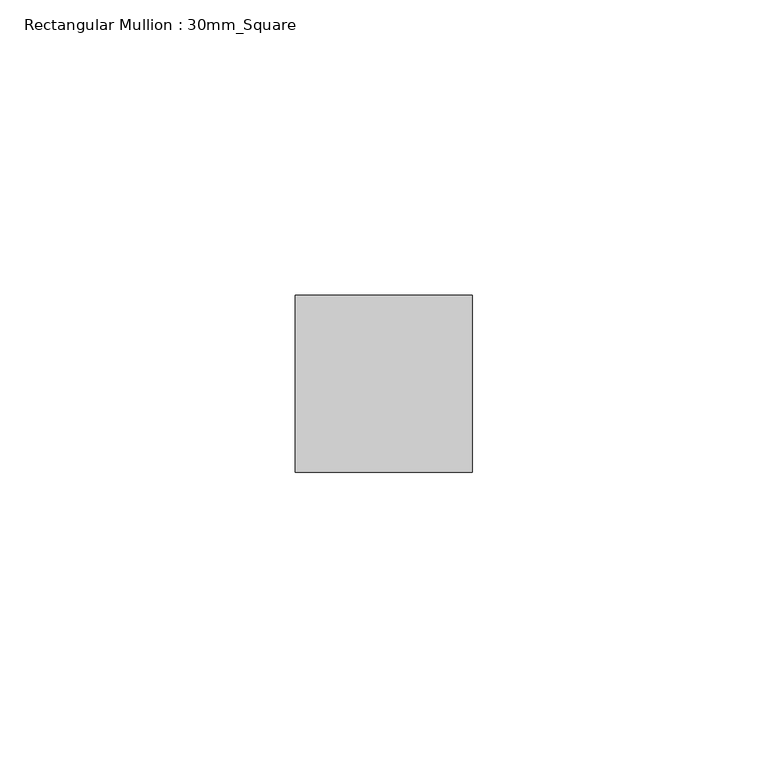
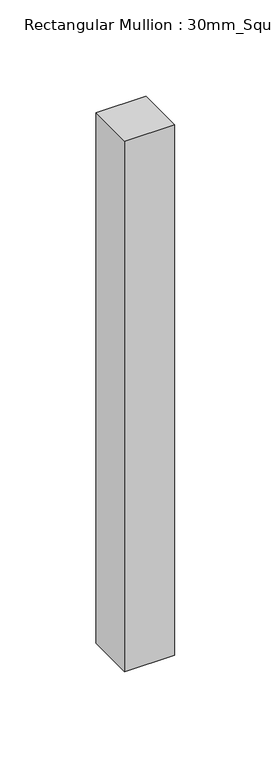
"""IFC4 building model written with IfcOpenShell, lengths in millimetres: member geometry, Rectangular Mullion : 30mm_Square."""

from ifc_helpers import new_model, si_unit, frame, origin, place, context, project, spatial, polyline, outline, extrude, source, transform, mapped, element, save


def rectangular_mullion_30mm_square_cec16e38(model_context):
    return source(origin(), model_context, "Body", "SweptSolid", [
        extrude(outline(polyline([(0.0, 15.0), (0.0, -15.0), (-30.0, -15.0), (-30.0, 15.0), (0.0, 15.0)])), frame((0.0, 0.0, -336.875), z_axis=(0.0, 0.0, 1.0), x_axis=(1.0, 0.0, 0.0)), (0.0, 0.0, 1.0), 336.875),
    ])


if __name__ == "__main__":
    model = new_model("IFC4")
    model_context = context("Model", 3, world=origin())
    ifc_project = project(units=[si_unit("LENGTHUNIT", "METRE", prefix="MILLI")], contexts=[model_context])
    site = spatial("IfcSite", under=ifc_project)
    building = spatial("IfcBuilding", under=site)
    placement = place(None, origin())
    rectangular_mullion_30mm_square_shape = rectangular_mullion_30mm_square_cec16e38(model_context)
    element("IfcMember", 1, ObjectType="Rectangular Mullion : 30mm_Square", at=placement, inside=building, context=model_context, shape_type="MappedRepresentation", body=[
        mapped(rectangular_mullion_30mm_square_shape, transform((0.0, 0.0, 0.0), x_axis=(1.0, 0.0, 0.0), y_axis=(0.0, 1.0, 0.0), z_axis=(0.0, 0.0, 1.0))),
    ])
    save(model, "model.ifc")

# Revit data of these elements
# Type "Rectangular Mullion : 30mm_Square"
#   Keynote = "H11"
#   built-in parameter 1007304 = 0.0984252 (stored number, unit not read)
#   built-in parameter 1007301 = 0.0492126 (stored number, unit not read)
#   built-in parameter 1007300 = 0.0492126 (stored number, unit not read)
# Element 1 (IfcMember, "Rectangular Mullion : 30mm_Square")
#   Materials on its faces: "Aluminium"
# Materials
#   "Aluminium": class "Metal", colour RGB 247 247 247, transparency 0, Description = "Aluminium 6061", Cost = 0
